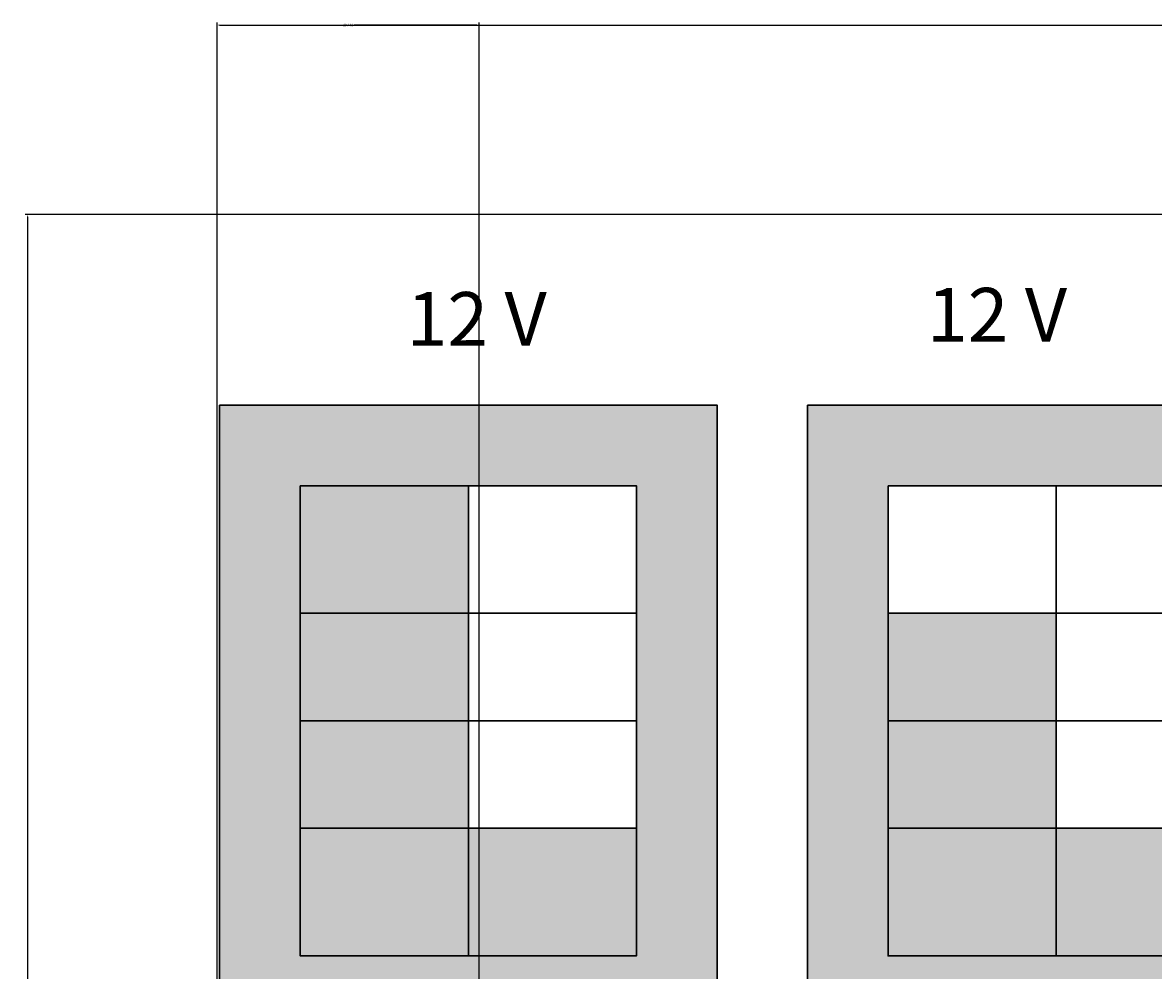
# Model space of a CAD drawing. Units: millimetres. Extents: x -8 to 285, y 5 to 221.
# Tile 14 of 30: x -8 to 76, y 150 to 221. Entities that reach past the tile are written whole.
import ezdxf

# ---------------------------------------------------------------- set-up
doc = ezdxf.new("R2010")
doc.units = ezdxf.units.MM
for name, color, linetype, lineweight in [('A-ANNO-DIMS', 2, 'Continuous', 18), ('E-ANNO-TEXT', 7, 'Continuous', 18), ('E-EQPM-PATT', 252, 'Continuous', 13), ('E-POWR-PV', 7, 'Continuous', 30)]:
    doc.layers.add(name, color=color, linetype=linetype, lineweight=lineweight)
doc.styles.get("Standard").update_dxf_attribs({"font": 'arial.ttf'})
doc.dimstyles.get("Standard").update_dxf_attribs({"dimtxt": 0.18, "dimasz": 0.18, "dimexe": 0.18, "dimexo": 0.0625, "dimgap": 0.09, "dimtad": 0, "dimtih": 1, "dimtoh": 1, "dimdec": 4, "dimzin": 0, "dimdsep": 46, "dimtxsty": 'Standard', "dimcen": 0.09, "dimadec": 0, "dimazin": 0, "dimtfac": 1, "dimtdec": 4, "dimtofl": 0, "dimtmove": 0, "dimatfit": 3, "dimfxl": 1, "dimtolj": 1, "dimtzin": 0, "dimarcsym": 0})

# ---------------------------------------------------------------- blocks, each defined once
blk = doc.blocks.new('PV-MODULE-12V')
for p, q in [((18.5, 41), (18.5, 6)), ((6, 31.5), (31, 31.5)), ((6, 23.5), (31, 23.5)), ((6, 15.5), (31, 15.5))]:
    blk.add_line(p, q)
for points in [[(0, 47), (37, 47), (37, 0), (0, 0)], [(6, 41), (31, 41), (31, 6), (6, 6)]]:
    blk.add_lwpolyline(points, close=True)
blk = doc.blocks.new('*D9')
at = {"layer": 'A-ANNO-DIMS', "color": 0, "lineweight": -2, "transparency": 16777216}
for p, q in [((6.672, 133.79), (6.672, 220.737)), ((6.852, 220.557), (138.33, 220.557)), ((270.739, 220.557), (139.262, 220.557)), ((270.919, 206.519), (270.919, 220.737))]:
    blk.add_line(p, q, dxfattribs=at)
at = {"layer": 'A-ANNO-DIMS', "color": 0, "transparency": 16777216}
for points in [[(6.852, 220.587), (6.852, 220.527), (6.672, 220.557)], [(270.739, 220.587), (270.739, 220.527), (270.919, 220.557)]]:
    blk.add_solid(points, dxfattribs=at)
at = {"layer": 'Defpoints', "color": 0, "transparency": 16777216}
for p in [(270.919, 220.557), (270.919, 206.457), (6.672, 133.727)]:
    blk.add_point(p, dxfattribs=at)
at = {"layer": 'A-ANNO-DIMS', "color": 0, "transparency": 16777216, "insert": (138.796, 220.557), "char_height": 0.18, "attachment_point": 5}
blk.add_mtext('\\A1;264.25', dxfattribs=at)
blk = doc.blocks.new('*D10')
at = {"layer": 'A-ANNO-DIMS', "color": 0, "lineweight": -2, "transparency": 16777216}
for p, q in [((145.103, 206.457), (-7.608, 206.457)), ((-7.428, 206.277), (-7.428, 113.161)), ((-7.428, 19.682), (-7.428, 112.797)), ((30.453, 19.502), (-7.608, 19.502))]:
    blk.add_line(p, q, dxfattribs=at)
at = {"layer": 'A-ANNO-DIMS', "color": 0, "transparency": 16777216}
for points in [[(-7.458, 206.277), (-7.398, 206.277), (-7.428, 206.457)], [(-7.458, 19.682), (-7.398, 19.682), (-7.428, 19.502)]]:
    blk.add_solid(points, dxfattribs=at)
at = {"layer": 'Defpoints', "color": 0, "transparency": 16777216}
for p in [(-7.428, 206.457), (145.165, 206.457), (30.516, 19.502)]:
    blk.add_point(p, dxfattribs=at)
at = {"layer": 'A-ANNO-DIMS', "color": 0, "transparency": 16777216, "insert": (-7.428, 112.979), "char_height": 0.18, "attachment_point": 5}
blk.add_mtext('\\A1;186.95', dxfattribs=at)
blk = doc.blocks.new('*D24')
at = {"layer": 'A-ANNO-DIMS', "color": 0, "lineweight": -2, "transparency": 16777216}
for p, q in [((6.672, 46.084), (6.672, 220.737)), ((6.852, 220.557), (15.959, 220.557)), ((25.975, 220.557), (16.869, 220.557)), ((26.155, 65.791), (26.155, 220.737))]:
    blk.add_line(p, q, dxfattribs=at)
at = {"layer": 'A-ANNO-DIMS', "color": 0, "transparency": 16777216}
for points in [[(6.852, 220.587), (6.852, 220.527), (6.672, 220.557)], [(25.975, 220.587), (25.975, 220.527), (26.155, 220.557)]]:
    blk.add_solid(points, dxfattribs=at)
at = {"layer": 'Defpoints', "color": 0, "transparency": 16777216}
for p in [(26.155, 220.557), (26.155, 65.728), (6.672, 46.021)]:
    blk.add_point(p, dxfattribs=at)
at = {"layer": 'A-ANNO-DIMS', "color": 0, "transparency": 16777216, "insert": (16.414, 220.557), "char_height": 0.18, "attachment_point": 5}
blk.add_mtext('\\A1;19.483', dxfattribs=at)

msp = doc.modelspace()

# ---------------------------------------------------------------- hatches: boundary and pattern name
at = {"layer": 'E-EQPM-PATT'}
h = msp.add_hatch(color=256, dxfattribs=at)
h.set_gradient(color2=(0, 0, 0), tint=1)
h.paths.add_polyline_path([(6.8535, 192.2715), (6.8535, 145.2715), (43.8535, 145.2715), (43.8535, 192.2715)])
h.paths.add_polyline_path([(37.8535, 186.2715), (37.8535, 151.2715), (12.8535, 151.2715), (12.8535, 186.2715)], flags=0)
h.paths.add_polyline_path([(50.5716, 145.2715), (87.5716, 145.2715), (87.5716, 192.2715), (50.5716, 192.2715)])
h.paths.add_polyline_path([(56.5716, 186.2715), (81.5716, 186.2715), (81.5716, 151.2715), (56.5716, 151.2715)], flags=0)
h.paths.add_polyline_path([(37.8535, 176.7715), (37.8535, 186.2715), (25.3535, 186.2715), (25.3535, 176.7715)], flags=0)
h.paths.add_polyline_path([(37.8535, 176.7715), (37.8535, 186.2715), (12.8535, 186.2715), (12.8535, 176.7715)], flags=0)
h.paths.add_polyline_path([(25.3535, 160.7715), (37.8535, 160.7715), (37.8535, 186.2715), (25.3535, 186.2715)], flags=0)
h.paths.add_polyline_path([(12.8535, 151.2715), (37.8535, 151.2715), (37.8535, 186.2715), (12.8535, 186.2715)], flags=16)
h.paths.add_polyline_path([(56.5716, 186.2715), (56.5716, 160.7715), (81.5716, 160.7715), (81.5716, 186.2715)], flags=0)
h.paths.add_polyline_path([(56.5716, 151.2715), (81.5716, 151.2715), (81.5716, 186.2715), (56.5716, 186.2715)], flags=16)
h = msp.add_hatch(color=256, dxfattribs=at)
h.set_gradient(color2=(0, 0, 0), tint=1)
h.paths.add_polyline_path([(25.3535, 186.2715), (12.8535, 186.2715), (12.8535, 176.7715), (25.3535, 176.7715)])
h.paths.add_polyline_path([(69.0716, 176.7715), (56.5716, 176.7715), (56.5716, 168.7715), (69.0716, 168.7715)])
h.paths.add_polyline_path([(69.0716, 168.7715), (56.5716, 168.7715), (56.5716, 160.7715), (69.0716, 160.7715)])
h.paths.add_polyline_path([(25.3535, 160.7715), (12.8535, 160.7715), (12.8535, 151.2715), (25.3535, 151.2715)])
h.paths.add_polyline_path([(81.5716, 160.7715), (69.0716, 160.7715), (69.0716, 151.2715), (81.5716, 151.2715)])

# ---------------------------------------------------------------- block references
at = {"layer": 'E-POWR-PV'}
for p in [(6.853, 145.271), (50.5711, 145.271)]:
    msp.add_blockref('PV-MODULE-12V', p, dxfattribs=at)

# ---------------------------------------------------------------- texts
at = {"layer": 'E-ANNO-TEXT', "char_height": 4, "attachment_point": 1}
for insert in [(59.462, 200.9913), (20.7625, 200.6799)]:
    msp.add_mtext_dynamic_manual_height_columns('12 V', width=28.779745, gutter_width=12.5, heights=[0], dxfattribs=dict(at, insert=insert))

# ---------------------------------------------------------------- dimensions: what is measured, and where the dimension line sits
at = {"layer": 'A-ANNO-DIMS'}
for base, p1, p2, override, picture, middle in [((270.9192, 220.5568), (6.6725, 133.7273), (270.9192, 206.4568), {"dimdec": 2, "dimlfac": 1, "dimrnd": 0, "dimzin": 0, "dimdsep": 46, "dimlunit": 2}, '*D9', (138.7958, 220.5568)), ((26.1554, 220.5568), (6.6725, 46.0211), (26.1554, 65.7282), {"dimdec": 3, "dimlfac": 1, "dimrnd": 0, "dimzin": 0, "dimdsep": 46, "dimlunit": 2}, '*D24', (16.4139, 220.5568))]:
    dim = msp.add_linear_dim(base=base, p1=p1, p2=p2, dimstyle='Standard', override=override, dxfattribs=at)
    dim.commit()
    dim.dimension.update_dxf_attribs({"geometry": picture, "text_midpoint": middle})
dim = msp.add_linear_dim(base=(-7.4275, 206.4568), p1=(30.516, 19.502), p2=(145.1651, 206.4568), angle=90, dimstyle='Standard', override={"dimdec": 2, "dimlfac": 1, "dimrnd": 0, "dimzin": 0, "dimdsep": 46, "dimlunit": 2}, dxfattribs=at)
dim.commit()
dim.dimension.update_dxf_attribs({"geometry": '*D10', "text_midpoint": (-7.4275, 112.9794)})

doc.saveas('drawing.dxf')
